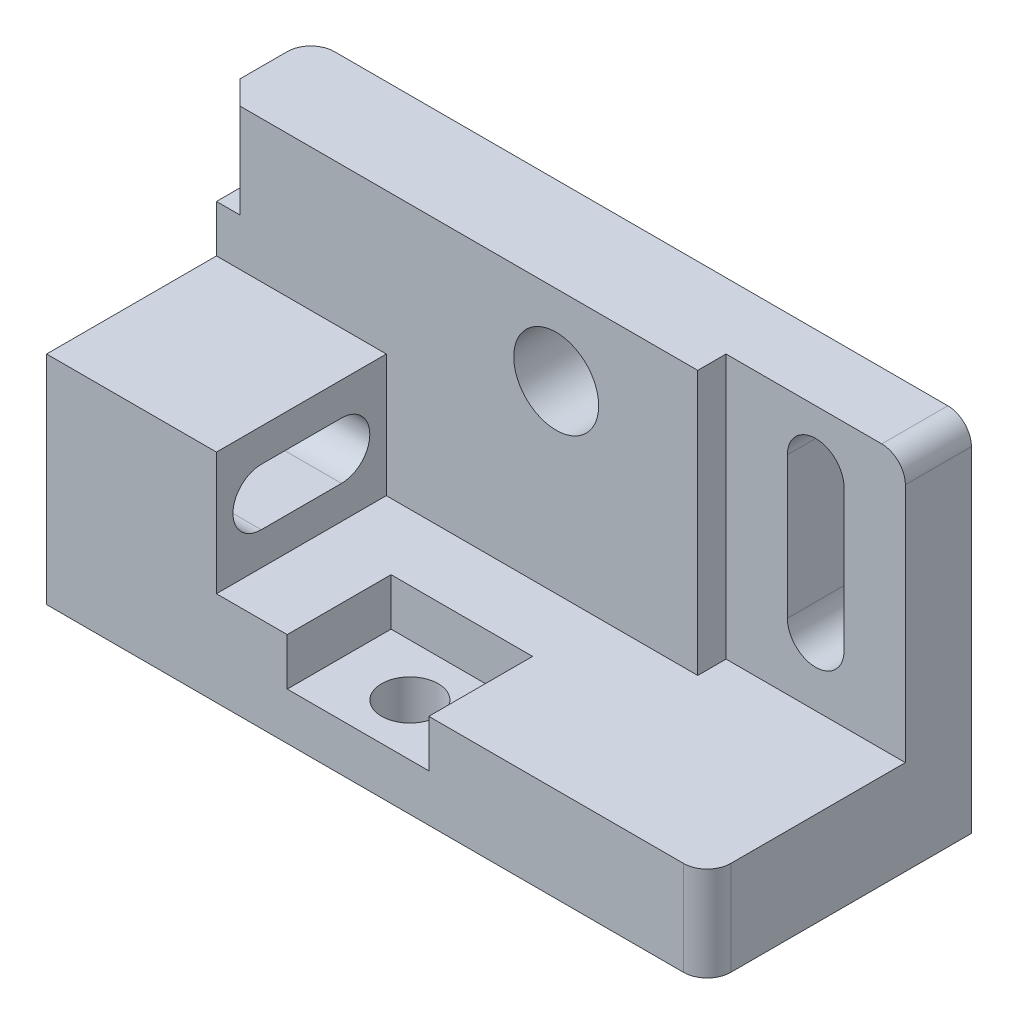
ISO-10303-21;
HEADER;
FILE_DESCRIPTION(('STEP AP214'),'2;1');
FILE_NAME('part.step','',(''),(''),'','','');
FILE_SCHEMA(('AUTOMOTIVE_DESIGN { 1 0 10303 214 1 1 1 1 }'));
ENDSEC;
DATA;
#1=APPLICATION_CONTEXT('core data for automotive mechanical design processes');
#2=APPLICATION_PROTOCOL_DEFINITION('international standard','automotive_design',2000,#1);
#3=PRODUCT_CONTEXT('',#1,'mechanical');
#4=PRODUCT('Part','Part','',(#3));
#5=PRODUCT_RELATED_PRODUCT_CATEGORY('part','',(#4));
#6=PRODUCT_DEFINITION_FORMATION('','',#4);
#7=PRODUCT_DEFINITION_CONTEXT('part definition',#1,'design');
#8=PRODUCT_DEFINITION('design','',#6,#7);
#9=PRODUCT_DEFINITION_SHAPE('','',#8);
#10=(LENGTH_UNIT() NAMED_UNIT(*) SI_UNIT(.MILLI.,.METRE.));
#11=(NAMED_UNIT(*) PLANE_ANGLE_UNIT() SI_UNIT($,.RADIAN.));
#12=(NAMED_UNIT(*) SI_UNIT($,.STERADIAN.) SOLID_ANGLE_UNIT());
#13=UNCERTAINTY_MEASURE_WITH_UNIT(LENGTH_MEASURE(1.E-05),#10,'distance_accuracy_value','');
#14=(GEOMETRIC_REPRESENTATION_CONTEXT(3) GLOBAL_UNCERTAINTY_ASSIGNED_CONTEXT((#13)) GLOBAL_UNIT_ASSIGNED_CONTEXT((#10,
#11,#12)) REPRESENTATION_CONTEXT('',''));
#15=CARTESIAN_POINT('',(0.,0.,0.));
#16=DIRECTION('',(0.,0.,1.));
#17=DIRECTION('',(1.,0.,0.));
#18=AXIS2_PLACEMENT_3D('',#15,#16,#17);
#19=CARTESIAN_POINT('',(-70.,38.,28.));
#20=DIRECTION('',(0.,-1.,0.));
#21=DIRECTION('',(0.,0.,-1.));
#22=AXIS2_PLACEMENT_3D('',#19,#20,#21);
#23=PLANE('',#22);
#24=DIRECTION('',(-1.,0.,0.));
#25=VECTOR('',#24,1.);
#26=CARTESIAN_POINT('',(70.,38.,-14.));
#27=LINE('',#26,#25);
#28=CARTESIAN_POINT('',(65.,38.,-14.));
#29=VERTEX_POINT('',#28);
#30=CARTESIAN_POINT('',(32.,38.,-14.));
#31=VERTEX_POINT('',#30);
#32=EDGE_CURVE('E337',#29,#31,#27,.T.);
#33=ORIENTED_EDGE('',*,*,#32,.F.);
#34=DIRECTION('',(0.,0.,-1.));
#35=VECTOR('',#34,1.);
#36=CARTESIAN_POINT('',(65.,38.,28.));
#37=LINE('',#36,#35);
#38=CARTESIAN_POINT('',(65.,38.,-28.));
#39=VERTEX_POINT('',#38);
#40=EDGE_CURVE('E447',#29,#39,#37,.T.);
#41=ORIENTED_EDGE('',*,*,#40,.T.);
#42=DIRECTION('',(-1.,0.,0.));
#43=VECTOR('',#42,1.);
#44=CARTESIAN_POINT('',(-70.,38.,-28.));
#45=LINE('',#44,#43);
#46=CARTESIAN_POINT('',(-65.,38.,-28.));
#47=VERTEX_POINT('',#46);
#48=EDGE_CURVE('E423',#39,#47,#45,.T.);
#49=ORIENTED_EDGE('',*,*,#48,.T.);
#50=CARTESIAN_POINT('',(-65.,38.,-23.));
#51=DIRECTION('',(0.,-1.,0.));
#52=DIRECTION('',(0.,0.,-1.));
#53=AXIS2_PLACEMENT_3D('',#50,#51,#52);
#54=CIRCLE('',#53,5.);
#55=CARTESIAN_POINT('',(-70.,38.,-23.));
#56=VERTEX_POINT('',#55);
#57=EDGE_CURVE('E271',#56,#47,#54,.T.);
#58=ORIENTED_EDGE('',*,*,#57,.F.);
#59=DIRECTION('',(0.,0.,-1.));
#60=VECTOR('',#59,1.);
#61=CARTESIAN_POINT('',(-70.,38.,28.));
#62=LINE('',#61,#60);
#63=CARTESIAN_POINT('',(-70.,38.,-13.));
#64=VERTEX_POINT('',#63);
#65=EDGE_CURVE('E431',#64,#56,#62,.T.);
#66=ORIENTED_EDGE('',*,*,#65,.F.);
#67=DIRECTION('',(-0.707106781186548,0.,-0.707106781186547));
#68=VECTOR('',#67,1.);
#69=CARTESIAN_POINT('',(-70.,38.,-13.));
#70=LINE('',#69,#68);
#71=CARTESIAN_POINT('',(-65.,38.,-8.));
#72=VERTEX_POINT('',#71);
#73=EDGE_CURVE('E279',#72,#64,#70,.T.);
#74=ORIENTED_EDGE('',*,*,#73,.F.);
#75=DIRECTION('',(-1.,0.,0.));
#76=VECTOR('',#75,1.);
#77=CARTESIAN_POINT('',(70.,38.,-8.));
#78=LINE('',#77,#76);
#79=CARTESIAN_POINT('',(32.,38.,-8.));
#80=VERTEX_POINT('',#79);
#81=EDGE_CURVE('E394',#80,#72,#78,.T.);
#82=ORIENTED_EDGE('',*,*,#81,.F.);
#83=DIRECTION('',(0.,0.,1.));
#84=VECTOR('',#83,1.);
#85=CARTESIAN_POINT('',(32.,38.,-14.));
#86=LINE('',#85,#84);
#87=EDGE_CURVE('E344',#31,#80,#86,.T.);
#88=ORIENTED_EDGE('',*,*,#87,.F.);
#89=EDGE_LOOP('',(#33,#41,#49,#58,#66,#74,#82,#88));
#90=FACE_BOUND('',#89,.T.);
#91=ADVANCED_FACE('F43',(#90),#23,.F.);
#92=CARTESIAN_POINT('',(70.,-38.,28.));
#93=DIRECTION('',(-1.,0.,0.));
#94=DIRECTION('',(0.,0.,1.));
#95=AXIS2_PLACEMENT_3D('',#92,#93,#94);
#96=PLANE('',#95);
#97=DIRECTION('',(0.,1.,0.));
#98=VECTOR('',#97,1.);
#99=CARTESIAN_POINT('',(70.,-38.,-28.));
#100=LINE('',#99,#98);
#101=CARTESIAN_POINT('',(70.,-38.,-28.));
#102=VERTEX_POINT('',#101);
#103=CARTESIAN_POINT('',(70.,33.,-28.));
#104=VERTEX_POINT('',#103);
#105=EDGE_CURVE('E409',#102,#104,#100,.T.);
#106=ORIENTED_EDGE('',*,*,#105,.T.);
#107=DIRECTION('',(0.,0.,-1.));
#108=VECTOR('',#107,1.);
#109=CARTESIAN_POINT('',(70.,33.,28.));
#110=LINE('',#109,#108);
#111=CARTESIAN_POINT('',(70.,33.,-14.));
#112=VERTEX_POINT('',#111);
#113=EDGE_CURVE('E453',#104,#112,#110,.F.);
#114=ORIENTED_EDGE('',*,*,#113,.T.);
#115=DIRECTION('',(0.,1.,0.));
#116=VECTOR('',#115,1.);
#117=CARTESIAN_POINT('',(70.,38.,-14.));
#118=LINE('',#117,#116);
#119=CARTESIAN_POINT('',(70.,-18.,-14.));
#120=VERTEX_POINT('',#119);
#121=EDGE_CURVE('E334',#120,#112,#118,.T.);
#122=ORIENTED_EDGE('',*,*,#121,.F.);
#123=DIRECTION('',(0.,0.,1.));
#124=VECTOR('',#123,1.);
#125=CARTESIAN_POINT('',(70.,-18.,-8.));
#126=LINE('',#125,#124);
#127=CARTESIAN_POINT('',(70.,-18.,23.));
#128=VERTEX_POINT('',#127);
#129=EDGE_CURVE('E404',#120,#128,#126,.T.);
#130=ORIENTED_EDGE('',*,*,#129,.T.);
#131=DIRECTION('',(0.,1.,0.));
#132=VECTOR('',#131,1.);
#133=CARTESIAN_POINT('',(70.,-38.,23.));
#134=LINE('',#133,#132);
#135=CARTESIAN_POINT('',(70.,-38.,23.));
#136=VERTEX_POINT('',#135);
#137=EDGE_CURVE('E452',#128,#136,#134,.F.);
#138=ORIENTED_EDGE('',*,*,#137,.T.);
#139=DIRECTION('',(0.,0.,-1.));
#140=VECTOR('',#139,1.);
#141=CARTESIAN_POINT('',(70.,-38.,28.));
#142=LINE('',#141,#140);
#143=EDGE_CURVE('E416',#136,#102,#142,.T.);
#144=ORIENTED_EDGE('',*,*,#143,.T.);
#145=EDGE_LOOP('',(#106,#114,#122,#130,#138,#144));
#146=FACE_BOUND('',#145,.T.);
#147=ADVANCED_FACE('F467',(#146),#96,.F.);
#148=CARTESIAN_POINT('',(-70.,-38.,28.));
#149=DIRECTION('',(1.,0.,0.));
#150=DIRECTION('',(0.,0.,-1.));
#151=AXIS2_PLACEMENT_3D('',#148,#149,#150);
#152=PLANE('',#151);
#153=DIRECTION('',(0.,0.,1.));
#154=VECTOR('',#153,1.);
#155=CARTESIAN_POINT('',(-70.,0.999999999999994,18.5));
#156=LINE('',#155,#154);
#157=CARTESIAN_POINT('',(-70.,0.999999999999994,1.5));
#158=VERTEX_POINT('',#157);
#159=CARTESIAN_POINT('',(-70.,0.999999999999994,18.5));
#160=VERTEX_POINT('',#159);
#161=EDGE_CURVE('E238',#158,#160,#156,.T.);
#162=ORIENTED_EDGE('',*,*,#161,.T.);
#163=CARTESIAN_POINT('',(-70.,-5.00000000000001,18.5));
#164=DIRECTION('',(1.,0.,0.));
#165=DIRECTION('',(0.,0.,-1.));
#166=AXIS2_PLACEMENT_3D('',#163,#164,#165);
#167=CIRCLE('',#166,6.);
#168=CARTESIAN_POINT('',(-70.,-11.,18.5));
#169=VERTEX_POINT('',#168);
#170=EDGE_CURVE('E235',#160,#169,#167,.T.);
#171=ORIENTED_EDGE('',*,*,#170,.T.);
#172=DIRECTION('',(0.,0.,-1.));
#173=VECTOR('',#172,1.);
#174=CARTESIAN_POINT('',(-70.,-11.,18.5));
#175=LINE('',#174,#173);
#176=CARTESIAN_POINT('',(-70.,-11.,1.5));
#177=VERTEX_POINT('',#176);
#178=EDGE_CURVE('E241',#169,#177,#175,.T.);
#179=ORIENTED_EDGE('',*,*,#178,.T.);
#180=CARTESIAN_POINT('',(-70.,-5.00000000000001,1.5));
#181=DIRECTION('',(1.,0.,0.));
#182=DIRECTION('',(0.,0.,-1.));
#183=AXIS2_PLACEMENT_3D('',#180,#181,#182);
#184=CIRCLE('',#183,6.);
#185=EDGE_CURVE('E248',#177,#158,#184,.T.);
#186=ORIENTED_EDGE('',*,*,#185,.T.);
#187=EDGE_LOOP('',(#162,#171,#179,#186));
#188=FACE_BOUND('',#187,.T.);
#189=DIRECTION('',(0.,0.,1.));
#190=VECTOR('',#189,1.);
#191=CARTESIAN_POINT('',(-70.,18.,-13.));
#192=LINE('',#191,#190);
#193=CARTESIAN_POINT('',(-70.,18.,-13.));
#194=VERTEX_POINT('',#193);
#195=CARTESIAN_POINT('',(-70.,18.,-8.));
#196=VERTEX_POINT('',#195);
#197=EDGE_CURVE('E274',#194,#196,#192,.T.);
#198=ORIENTED_EDGE('',*,*,#197,.F.);
#199=DIRECTION('',(0.,1.,0.));
#200=VECTOR('',#199,1.);
#201=CARTESIAN_POINT('',(-70.,18.,-13.));
#202=LINE('',#201,#200);
#203=EDGE_CURVE('E287',#194,#64,#202,.T.);
#204=ORIENTED_EDGE('',*,*,#203,.T.);
#205=ORIENTED_EDGE('',*,*,#65,.T.);
#206=DIRECTION('',(0.,1.,0.));
#207=VECTOR('',#206,1.);
#208=CARTESIAN_POINT('',(-70.,18.,-23.));
#209=LINE('',#208,#207);
#210=CARTESIAN_POINT('',(-70.,18.,-23.));
#211=VERTEX_POINT('',#210);
#212=EDGE_CURVE('E283',#211,#56,#209,.T.);
#213=ORIENTED_EDGE('',*,*,#212,.F.);
#214=DIRECTION('',(0.,0.,1.));
#215=VECTOR('',#214,1.);
#216=CARTESIAN_POINT('',(-70.,18.,-23.));
#217=LINE('',#216,#215);
#218=CARTESIAN_POINT('',(-70.,18.,-28.));
#219=VERTEX_POINT('',#218);
#220=EDGE_CURVE('E293',#219,#211,#217,.T.);
#221=ORIENTED_EDGE('',*,*,#220,.F.);
#222=DIRECTION('',(0.,-1.,0.));
#223=VECTOR('',#222,1.);
#224=CARTESIAN_POINT('',(-70.,-38.,-28.));
#225=LINE('',#224,#223);
#226=CARTESIAN_POINT('',(-70.,-38.,-28.));
#227=VERTEX_POINT('',#226);
#228=EDGE_CURVE('E421',#219,#227,#225,.T.);
#229=ORIENTED_EDGE('',*,*,#228,.T.);
#230=DIRECTION('',(0.,0.,-1.));
#231=VECTOR('',#230,1.);
#232=CARTESIAN_POINT('',(-70.,-38.,28.));
#233=LINE('',#232,#231);
#234=CARTESIAN_POINT('',(-70.,-38.,28.));
#235=VERTEX_POINT('',#234);
#236=EDGE_CURVE('E428',#235,#227,#233,.T.);
#237=ORIENTED_EDGE('',*,*,#236,.F.);
#238=DIRECTION('',(0.,-1.,0.));
#239=VECTOR('',#238,1.);
#240=CARTESIAN_POINT('',(-70.,-38.,28.));
#241=LINE('',#240,#239);
#242=CARTESIAN_POINT('',(-70.,7.99999999999999,28.));
#243=VERTEX_POINT('',#242);
#244=EDGE_CURVE('E413',#243,#235,#241,.T.);
#245=ORIENTED_EDGE('',*,*,#244,.F.);
#246=DIRECTION('',(0.,0.,1.));
#247=VECTOR('',#246,1.);
#248=CARTESIAN_POINT('',(-70.,7.99999999999999,-8.));
#249=LINE('',#248,#247);
#250=CARTESIAN_POINT('',(-70.,7.99999999999999,-8.));
#251=VERTEX_POINT('',#250);
#252=EDGE_CURVE('E393',#251,#243,#249,.T.);
#253=ORIENTED_EDGE('',*,*,#252,.F.);
#254=DIRECTION('',(0.,-1.,0.));
#255=VECTOR('',#254,1.);
#256=CARTESIAN_POINT('',(-70.,38.,-8.));
#257=LINE('',#256,#255);
#258=EDGE_CURVE('E379',#196,#251,#257,.T.);
#259=ORIENTED_EDGE('',*,*,#258,.F.);
#260=EDGE_LOOP('',(#198,#204,#205,#213,#221,#229,#237,#245,#253,#259));
#261=FACE_BOUND('',#260,.T.);
#262=ADVANCED_FACE('F246',(#188,#261),#152,.F.);
#263=CARTESIAN_POINT('',(-70.,-38.,28.));
#264=DIRECTION('',(0.,1.,0.));
#265=DIRECTION('',(0.,0.,1.));
#266=AXIS2_PLACEMENT_3D('',#263,#264,#265);
#267=PLANE('',#266);
#268=CARTESIAN_POINT('',(-4.00000000000002,-38.,17.));
#269=DIRECTION('',(0.,1.,0.));
#270=DIRECTION('',(0.,0.,1.));
#271=AXIS2_PLACEMENT_3D('',#268,#269,#270);
#272=CIRCLE('',#271,6.);
#273=CARTESIAN_POINT('',(-4.00000000000002,-38.,23.));
#274=VERTEX_POINT('',#273);
#275=EDGE_CURVE('E259',#274,#274,#272,.T.);
#276=ORIENTED_EDGE('',*,*,#275,.T.);
#277=EDGE_LOOP('',(#276));
#278=FACE_BOUND('',#277,.T.);
#279=ORIENTED_EDGE('',*,*,#143,.F.);
#280=CARTESIAN_POINT('',(65.,-38.,23.));
#281=DIRECTION('',(0.,1.,0.));
#282=DIRECTION('',(0.,0.,1.));
#283=AXIS2_PLACEMENT_3D('',#280,#281,#282);
#284=CIRCLE('',#283,5.);
#285=CARTESIAN_POINT('',(65.,-38.,28.));
#286=VERTEX_POINT('',#285);
#287=EDGE_CURVE('E11',#136,#286,#284,.F.);
#288=ORIENTED_EDGE('',*,*,#287,.T.);
#289=DIRECTION('',(1.,0.,0.));
#290=VECTOR('',#289,1.);
#291=CARTESIAN_POINT('',(-70.,-38.,28.));
#292=LINE('',#291,#290);
#293=EDGE_CURVE('E411',#235,#286,#292,.T.);
#294=ORIENTED_EDGE('',*,*,#293,.F.);
#295=ORIENTED_EDGE('',*,*,#236,.T.);
#296=DIRECTION('',(1.,0.,0.));
#297=VECTOR('',#296,1.);
#298=CARTESIAN_POINT('',(-70.,-38.,-28.));
#299=LINE('',#298,#297);
#300=EDGE_CURVE('E418',#227,#102,#299,.T.);
#301=ORIENTED_EDGE('',*,*,#300,.T.);
#302=EDGE_LOOP('',(#279,#288,#294,#295,#301));
#303=FACE_BOUND('',#302,.T.);
#304=ADVANCED_FACE('F471',(#278,#303),#267,.F.);
#305=CARTESIAN_POINT('',(0.,0.,28.));
#306=DIRECTION('',(0.,0.,-1.));
#307=DIRECTION('',(-1.,0.,0.));
#308=AXIS2_PLACEMENT_3D('',#305,#306,#307);
#309=PLANE('',#308);
#310=ORIENTED_EDGE('',*,*,#293,.T.);
#311=DIRECTION('',(0.,1.,0.));
#312=VECTOR('',#311,1.);
#313=CARTESIAN_POINT('',(65.,0.,28.));
#314=LINE('',#313,#312);
#315=CARTESIAN_POINT('',(65.,-18.,28.));
#316=VERTEX_POINT('',#315);
#317=EDGE_CURVE('E460',#286,#316,#314,.T.);
#318=ORIENTED_EDGE('',*,*,#317,.T.);
#319=DIRECTION('',(1.,0.,0.));
#320=VECTOR('',#319,1.);
#321=CARTESIAN_POINT('',(-34.,-18.,28.));
#322=LINE('',#321,#320);
#323=CARTESIAN_POINT('',(11.,-18.,28.));
#324=VERTEX_POINT('',#323);
#325=EDGE_CURVE('E402',#324,#316,#322,.T.);
#326=ORIENTED_EDGE('',*,*,#325,.F.);
#327=DIRECTION('',(0.,1.,0.));
#328=VECTOR('',#327,1.);
#329=CARTESIAN_POINT('',(11.,-28.,28.));
#330=LINE('',#329,#328);
#331=CARTESIAN_POINT('',(11.,-28.,28.));
#332=VERTEX_POINT('',#331);
#333=EDGE_CURVE('E367',#332,#324,#330,.T.);
#334=ORIENTED_EDGE('',*,*,#333,.F.);
#335=DIRECTION('',(1.,0.,0.));
#336=VECTOR('',#335,1.);
#337=CARTESIAN_POINT('',(11.,-28.,28.));
#338=LINE('',#337,#336);
#339=CARTESIAN_POINT('',(-19.,-28.,28.));
#340=VERTEX_POINT('',#339);
#341=EDGE_CURVE('E363',#340,#332,#338,.T.);
#342=ORIENTED_EDGE('',*,*,#341,.F.);
#343=DIRECTION('',(0.,1.,0.));
#344=VECTOR('',#343,1.);
#345=CARTESIAN_POINT('',(-19.,-28.,28.));
#346=LINE('',#345,#344);
#347=CARTESIAN_POINT('',(-19.,-18.,28.));
#348=VERTEX_POINT('',#347);
#349=EDGE_CURVE('E373',#340,#348,#346,.T.);
#350=ORIENTED_EDGE('',*,*,#349,.T.);
#351=CARTESIAN_POINT('',(-34.,-18.,28.));
#352=VERTEX_POINT('',#351);
#353=EDGE_CURVE('E382',#352,#348,#322,.T.);
#354=ORIENTED_EDGE('',*,*,#353,.F.);
#355=DIRECTION('',(0.,-1.,0.));
#356=VECTOR('',#355,1.);
#357=CARTESIAN_POINT('',(-34.,7.99999999999999,28.));
#358=LINE('',#357,#356);
#359=CARTESIAN_POINT('',(-34.,7.99999999999999,28.));
#360=VERTEX_POINT('',#359);
#361=EDGE_CURVE('E398',#360,#352,#358,.T.);
#362=ORIENTED_EDGE('',*,*,#361,.F.);
#363=DIRECTION('',(1.,0.,0.));
#364=VECTOR('',#363,1.);
#365=CARTESIAN_POINT('',(-70.,7.99999999999999,28.));
#366=LINE('',#365,#364);
#367=EDGE_CURVE('E375',#243,#360,#366,.T.);
#368=ORIENTED_EDGE('',*,*,#367,.F.);
#369=ORIENTED_EDGE('',*,*,#244,.T.);
#370=EDGE_LOOP('',(#310,#318,#326,#334,#342,#350,#354,#362,#368,#369));
#371=FACE_BOUND('',#370,.T.);
#372=ADVANCED_FACE('F468',(#371),#309,.F.);
#373=CARTESIAN_POINT('',(0.,0.,-28.));
#374=DIRECTION('',(0.,0.,-1.));
#375=DIRECTION('',(-1.,0.,0.));
#376=AXIS2_PLACEMENT_3D('',#373,#374,#375);
#377=PLANE('',#376);
#378=ORIENTED_EDGE('',*,*,#48,.F.);
#379=CARTESIAN_POINT('',(65.,33.,-28.));
#380=DIRECTION('',(0.,0.,-1.));
#381=DIRECTION('',(-1.,0.,0.));
#382=AXIS2_PLACEMENT_3D('',#379,#380,#381);
#383=CIRCLE('',#382,5.);
#384=EDGE_CURVE('E446',#39,#104,#383,.T.);
#385=ORIENTED_EDGE('',*,*,#384,.T.);
#386=ORIENTED_EDGE('',*,*,#105,.F.);
#387=ORIENTED_EDGE('',*,*,#300,.F.);
#388=ORIENTED_EDGE('',*,*,#228,.F.);
#389=DIRECTION('',(-1.,0.,0.));
#390=VECTOR('',#389,1.);
#391=CARTESIAN_POINT('',(-70.,18.,-28.));
#392=LINE('',#391,#390);
#393=CARTESIAN_POINT('',(-65.,18.,-28.));
#394=VERTEX_POINT('',#393);
#395=EDGE_CURVE('E291',#394,#219,#392,.T.);
#396=ORIENTED_EDGE('',*,*,#395,.F.);
#397=DIRECTION('',(0.,1.,0.));
#398=VECTOR('',#397,1.);
#399=CARTESIAN_POINT('',(-65.,18.,-28.));
#400=LINE('',#399,#398);
#401=EDGE_CURVE('E300',#394,#47,#400,.T.);
#402=ORIENTED_EDGE('',*,*,#401,.T.);
#403=EDGE_LOOP('',(#378,#385,#386,#387,#388,#396,#402));
#404=FACE_BOUND('',#403,.T.);
#405=CARTESIAN_POINT('',(1.99999999999999,21.,-28.));
#406=DIRECTION('',(0.,0.,1.));
#407=DIRECTION('',(1.,0.,0.));
#408=AXIS2_PLACEMENT_3D('',#405,#406,#407);
#409=CIRCLE('',#408,9.);
#410=CARTESIAN_POINT('',(11.,21.,-28.));
#411=VERTEX_POINT('',#410);
#412=EDGE_CURVE('E304',#411,#411,#409,.T.);
#413=ORIENTED_EDGE('',*,*,#412,.T.);
#414=EDGE_LOOP('',(#413));
#415=FACE_BOUND('',#414,.T.);
#416=CARTESIAN_POINT('',(51.,-4.00000000000001,-28.));
#417=DIRECTION('',(0.,0.,1.));
#418=DIRECTION('',(1.,0.,0.));
#419=AXIS2_PLACEMENT_3D('',#416,#417,#418);
#420=CIRCLE('',#419,6.);
#421=CARTESIAN_POINT('',(45.,-4.00000000000001,-28.));
#422=VERTEX_POINT('',#421);
#423=CARTESIAN_POINT('',(57.,-4.00000000000001,-28.));
#424=VERTEX_POINT('',#423);
#425=EDGE_CURVE('E289',#422,#424,#420,.T.);
#426=ORIENTED_EDGE('',*,*,#425,.T.);
#427=DIRECTION('',(0.,1.,0.));
#428=VECTOR('',#427,1.);
#429=CARTESIAN_POINT('',(57.,-4.00000000000001,-28.));
#430=LINE('',#429,#428);
#431=CARTESIAN_POINT('',(57.,26.,-28.));
#432=VERTEX_POINT('',#431);
#433=EDGE_CURVE('E314',#424,#432,#430,.T.);
#434=ORIENTED_EDGE('',*,*,#433,.T.);
#435=CARTESIAN_POINT('',(51.,26.,-28.));
#436=DIRECTION('',(0.,0.,1.));
#437=DIRECTION('',(1.,0.,0.));
#438=AXIS2_PLACEMENT_3D('',#435,#436,#437);
#439=CIRCLE('',#438,6.);
#440=CARTESIAN_POINT('',(45.,26.,-28.));
#441=VERTEX_POINT('',#440);
#442=EDGE_CURVE('E320',#432,#441,#439,.T.);
#443=ORIENTED_EDGE('',*,*,#442,.T.);
#444=DIRECTION('',(0.,-1.,0.));
#445=VECTOR('',#444,1.);
#446=CARTESIAN_POINT('',(45.,-4.00000000000001,-28.));
#447=LINE('',#446,#445);
#448=EDGE_CURVE('E319',#441,#422,#447,.T.);
#449=ORIENTED_EDGE('',*,*,#448,.T.);
#450=EDGE_LOOP('',(#426,#434,#443,#449));
#451=FACE_BOUND('',#450,.T.);
#452=ADVANCED_FACE('F479',(#404,#415,#451),#377,.T.);
#453=CARTESIAN_POINT('',(-34.,-18.,-8.));
#454=DIRECTION('',(0.,-1.,0.));
#455=DIRECTION('',(0.,0.,-1.));
#456=AXIS2_PLACEMENT_3D('',#453,#454,#455);
#457=PLANE('',#456);
#458=ORIENTED_EDGE('',*,*,#325,.T.);
#459=CARTESIAN_POINT('',(65.,-18.,23.));
#460=DIRECTION('',(0.,-1.,0.));
#461=DIRECTION('',(0.,0.,-1.));
#462=AXIS2_PLACEMENT_3D('',#459,#460,#461);
#463=CIRCLE('',#462,5.);
#464=EDGE_CURVE('E51',#316,#128,#463,.F.);
#465=ORIENTED_EDGE('',*,*,#464,.T.);
#466=ORIENTED_EDGE('',*,*,#129,.F.);
#467=DIRECTION('',(1.,0.,0.));
#468=VECTOR('',#467,1.);
#469=CARTESIAN_POINT('',(70.,-18.,-14.));
#470=LINE('',#469,#468);
#471=CARTESIAN_POINT('',(32.,-18.,-14.));
#472=VERTEX_POINT('',#471);
#473=EDGE_CURVE('E342',#472,#120,#470,.T.);
#474=ORIENTED_EDGE('',*,*,#473,.F.);
#475=DIRECTION('',(0.,0.,1.));
#476=VECTOR('',#475,1.);
#477=CARTESIAN_POINT('',(32.,-18.,-14.));
#478=LINE('',#477,#476);
#479=CARTESIAN_POINT('',(32.,-18.,-8.));
#480=VERTEX_POINT('',#479);
#481=EDGE_CURVE('E350',#472,#480,#478,.T.);
#482=ORIENTED_EDGE('',*,*,#481,.T.);
#483=DIRECTION('',(1.,0.,0.));
#484=VECTOR('',#483,1.);
#485=CARTESIAN_POINT('',(-34.,-18.,-8.));
#486=LINE('',#485,#484);
#487=CARTESIAN_POINT('',(-34.,-18.,-8.));
#488=VERTEX_POINT('',#487);
#489=EDGE_CURVE('E386',#488,#480,#486,.T.);
#490=ORIENTED_EDGE('',*,*,#489,.F.);
#491=DIRECTION('',(0.,0.,1.));
#492=VECTOR('',#491,1.);
#493=CARTESIAN_POINT('',(-34.,-18.,-8.));
#494=LINE('',#493,#492);
#495=EDGE_CURVE('E410',#488,#352,#494,.T.);
#496=ORIENTED_EDGE('',*,*,#495,.T.);
#497=ORIENTED_EDGE('',*,*,#353,.T.);
#498=DIRECTION('',(0.,0.,1.));
#499=VECTOR('',#498,1.);
#500=CARTESIAN_POINT('',(-19.,-18.,28.));
#501=LINE('',#500,#499);
#502=CARTESIAN_POINT('',(-19.,-18.,6.00000000000001));
#503=VERTEX_POINT('',#502);
#504=EDGE_CURVE('E353',#503,#348,#501,.T.);
#505=ORIENTED_EDGE('',*,*,#504,.F.);
#506=DIRECTION('',(-1.,0.,0.));
#507=VECTOR('',#506,1.);
#508=CARTESIAN_POINT('',(11.,-18.,6.));
#509=LINE('',#508,#507);
#510=CARTESIAN_POINT('',(11.,-18.,6.));
#511=VERTEX_POINT('',#510);
#512=EDGE_CURVE('E368',#511,#503,#509,.T.);
#513=ORIENTED_EDGE('',*,*,#512,.F.);
#514=DIRECTION('',(0.,0.,-1.));
#515=VECTOR('',#514,1.);
#516=CARTESIAN_POINT('',(11.,-18.,28.));
#517=LINE('',#516,#515);
#518=EDGE_CURVE('E349',#324,#511,#517,.T.);
#519=ORIENTED_EDGE('',*,*,#518,.F.);
#520=EDGE_LOOP('',(#458,#465,#466,#474,#482,#490,#496,#497,#505,#513,#519));
#521=FACE_BOUND('',#520,.T.);
#522=ADVANCED_FACE('F458',(#521),#457,.F.);
#523=CARTESIAN_POINT('',(-34.,7.99999999999999,-8.));
#524=DIRECTION('',(-1.,0.,0.));
#525=DIRECTION('',(0.,0.,1.));
#526=AXIS2_PLACEMENT_3D('',#523,#524,#525);
#527=PLANE('',#526);
#528=DIRECTION('',(0.,0.,-1.));
#529=VECTOR('',#528,1.);
#530=CARTESIAN_POINT('',(-34.,-11.,18.5));
#531=LINE('',#530,#529);
#532=CARTESIAN_POINT('',(-34.,-11.,18.5));
#533=VERTEX_POINT('',#532);
#534=CARTESIAN_POINT('',(-34.,-11.,1.5));
#535=VERTEX_POINT('',#534);
#536=EDGE_CURVE('E264',#533,#535,#531,.T.);
#537=ORIENTED_EDGE('',*,*,#536,.F.);
#538=CARTESIAN_POINT('',(-34.,-5.00000000000001,18.5));
#539=DIRECTION('',(1.,0.,0.));
#540=DIRECTION('',(0.,0.,-1.));
#541=AXIS2_PLACEMENT_3D('',#538,#539,#540);
#542=CIRCLE('',#541,6.);
#543=CARTESIAN_POINT('',(-34.,0.999999999999994,18.5));
#544=VERTEX_POINT('',#543);
#545=EDGE_CURVE('E231',#544,#533,#542,.T.);
#546=ORIENTED_EDGE('',*,*,#545,.F.);
#547=DIRECTION('',(0.,0.,1.));
#548=VECTOR('',#547,1.);
#549=CARTESIAN_POINT('',(-34.,0.999999999999994,18.5));
#550=LINE('',#549,#548);
#551=CARTESIAN_POINT('',(-34.,0.999999999999994,1.5));
#552=VERTEX_POINT('',#551);
#553=EDGE_CURVE('E251',#552,#544,#550,.T.);
#554=ORIENTED_EDGE('',*,*,#553,.F.);
#555=CARTESIAN_POINT('',(-34.,-5.00000000000001,1.5));
#556=DIRECTION('',(1.,0.,0.));
#557=DIRECTION('',(0.,0.,-1.));
#558=AXIS2_PLACEMENT_3D('',#555,#556,#557);
#559=CIRCLE('',#558,6.);
#560=EDGE_CURVE('E258',#535,#552,#559,.T.);
#561=ORIENTED_EDGE('',*,*,#560,.F.);
#562=EDGE_LOOP('',(#537,#546,#554,#561));
#563=FACE_BOUND('',#562,.T.);
#564=ORIENTED_EDGE('',*,*,#361,.T.);
#565=ORIENTED_EDGE('',*,*,#495,.F.);
#566=DIRECTION('',(0.,-1.,0.));
#567=VECTOR('',#566,1.);
#568=CARTESIAN_POINT('',(-34.,7.99999999999999,-8.));
#569=LINE('',#568,#567);
#570=CARTESIAN_POINT('',(-34.,7.99999999999999,-8.));
#571=VERTEX_POINT('',#570);
#572=EDGE_CURVE('E387',#571,#488,#569,.T.);
#573=ORIENTED_EDGE('',*,*,#572,.F.);
#574=DIRECTION('',(0.,0.,1.));
#575=VECTOR('',#574,1.);
#576=CARTESIAN_POINT('',(-34.,7.99999999999999,-8.));
#577=LINE('',#576,#575);
#578=EDGE_CURVE('E408',#571,#360,#577,.T.);
#579=ORIENTED_EDGE('',*,*,#578,.T.);
#580=EDGE_LOOP('',(#564,#565,#573,#579));
#581=FACE_BOUND('',#580,.T.);
#582=ADVANCED_FACE('F508',(#563,#581),#527,.F.);
#583=CARTESIAN_POINT('',(-70.,7.99999999999999,-8.));
#584=DIRECTION('',(0.,-1.,0.));
#585=DIRECTION('',(0.,0.,-1.));
#586=AXIS2_PLACEMENT_3D('',#583,#584,#585);
#587=PLANE('',#586);
#588=ORIENTED_EDGE('',*,*,#367,.T.);
#589=ORIENTED_EDGE('',*,*,#578,.F.);
#590=DIRECTION('',(1.,0.,0.));
#591=VECTOR('',#590,1.);
#592=CARTESIAN_POINT('',(-70.,7.99999999999999,-8.));
#593=LINE('',#592,#591);
#594=EDGE_CURVE('E385',#251,#571,#593,.T.);
#595=ORIENTED_EDGE('',*,*,#594,.F.);
#596=ORIENTED_EDGE('',*,*,#252,.T.);
#597=EDGE_LOOP('',(#588,#589,#595,#596));
#598=FACE_BOUND('',#597,.T.);
#599=ADVANCED_FACE('F530',(#598),#587,.F.);
#600=CARTESIAN_POINT('',(0.,0.,-8.));
#601=DIRECTION('',(0.,0.,1.));
#602=DIRECTION('',(1.,0.,0.));
#603=AXIS2_PLACEMENT_3D('',#600,#601,#602);
#604=PLANE('',#603);
#605=DIRECTION('',(0.,1.,0.));
#606=VECTOR('',#605,1.);
#607=CARTESIAN_POINT('',(-65.,18.,-8.));
#608=LINE('',#607,#606);
#609=CARTESIAN_POINT('',(-65.,18.,-8.));
#610=VERTEX_POINT('',#609);
#611=EDGE_CURVE('E285',#610,#72,#608,.T.);
#612=ORIENTED_EDGE('',*,*,#611,.F.);
#613=DIRECTION('',(1.,0.,0.));
#614=VECTOR('',#613,1.);
#615=CARTESIAN_POINT('',(-70.,18.,-8.));
#616=LINE('',#615,#614);
#617=EDGE_CURVE('E280',#196,#610,#616,.T.);
#618=ORIENTED_EDGE('',*,*,#617,.F.);
#619=ORIENTED_EDGE('',*,*,#258,.T.);
#620=ORIENTED_EDGE('',*,*,#594,.T.);
#621=ORIENTED_EDGE('',*,*,#572,.T.);
#622=ORIENTED_EDGE('',*,*,#489,.T.);
#623=DIRECTION('',(0.,-1.,0.));
#624=VECTOR('',#623,1.);
#625=CARTESIAN_POINT('',(32.,38.,-8.));
#626=LINE('',#625,#624);
#627=EDGE_CURVE('E307',#80,#480,#626,.T.);
#628=ORIENTED_EDGE('',*,*,#627,.F.);
#629=ORIENTED_EDGE('',*,*,#81,.T.);
#630=EDGE_LOOP('',(#612,#618,#619,#620,#621,#622,#628,#629));
#631=FACE_BOUND('',#630,.T.);
#632=CARTESIAN_POINT('',(1.99999999999999,21.,-8.));
#633=DIRECTION('',(0.,0.,1.));
#634=DIRECTION('',(1.,0.,0.));
#635=AXIS2_PLACEMENT_3D('',#632,#633,#634);
#636=CIRCLE('',#635,9.);
#637=CARTESIAN_POINT('',(11.,21.,-8.));
#638=VERTEX_POINT('',#637);
#639=EDGE_CURVE('E306',#638,#638,#636,.T.);
#640=ORIENTED_EDGE('',*,*,#639,.F.);
#641=EDGE_LOOP('',(#640));
#642=FACE_BOUND('',#641,.T.);
#643=ADVANCED_FACE('F498',(#631,#642),#604,.T.);
#644=CARTESIAN_POINT('',(11.,-28.,28.));
#645=DIRECTION('',(1.,0.,0.));
#646=DIRECTION('',(0.,0.,-1.));
#647=AXIS2_PLACEMENT_3D('',#644,#645,#646);
#648=PLANE('',#647);
#649=ORIENTED_EDGE('',*,*,#518,.T.);
#650=DIRECTION('',(0.,1.,0.));
#651=VECTOR('',#650,1.);
#652=CARTESIAN_POINT('',(11.,-28.,6.));
#653=LINE('',#652,#651);
#654=CARTESIAN_POINT('',(11.,-28.,6.));
#655=VERTEX_POINT('',#654);
#656=EDGE_CURVE('E365',#655,#511,#653,.T.);
#657=ORIENTED_EDGE('',*,*,#656,.F.);
#658=DIRECTION('',(0.,0.,-1.));
#659=VECTOR('',#658,1.);
#660=CARTESIAN_POINT('',(11.,-28.,28.));
#661=LINE('',#660,#659);
#662=EDGE_CURVE('E352',#332,#655,#661,.T.);
#663=ORIENTED_EDGE('',*,*,#662,.F.);
#664=ORIENTED_EDGE('',*,*,#333,.T.);
#665=EDGE_LOOP('',(#649,#657,#663,#664));
#666=FACE_BOUND('',#665,.T.);
#667=ADVANCED_FACE('F518',(#666),#648,.F.);
#668=CARTESIAN_POINT('',(-19.,-28.,28.));
#669=DIRECTION('',(-1.,0.,0.));
#670=DIRECTION('',(0.,0.,1.));
#671=AXIS2_PLACEMENT_3D('',#668,#669,#670);
#672=PLANE('',#671);
#673=ORIENTED_EDGE('',*,*,#504,.T.);
#674=ORIENTED_EDGE('',*,*,#349,.F.);
#675=DIRECTION('',(0.,0.,1.));
#676=VECTOR('',#675,1.);
#677=CARTESIAN_POINT('',(-19.,-28.,28.));
#678=LINE('',#677,#676);
#679=CARTESIAN_POINT('',(-19.,-28.,6.00000000000001));
#680=VERTEX_POINT('',#679);
#681=EDGE_CURVE('E358',#680,#340,#678,.T.);
#682=ORIENTED_EDGE('',*,*,#681,.F.);
#683=DIRECTION('',(0.,1.,0.));
#684=VECTOR('',#683,1.);
#685=CARTESIAN_POINT('',(-19.,-28.,6.00000000000001));
#686=LINE('',#685,#684);
#687=EDGE_CURVE('E376',#680,#503,#686,.T.);
#688=ORIENTED_EDGE('',*,*,#687,.T.);
#689=EDGE_LOOP('',(#673,#674,#682,#688));
#690=FACE_BOUND('',#689,.T.);
#691=ADVANCED_FACE('F515',(#690),#672,.F.);
#692=CARTESIAN_POINT('',(11.,-28.,6.));
#693=DIRECTION('',(0.,0.,-1.));
#694=DIRECTION('',(-1.,0.,0.));
#695=AXIS2_PLACEMENT_3D('',#692,#693,#694);
#696=PLANE('',#695);
#697=ORIENTED_EDGE('',*,*,#512,.T.);
#698=ORIENTED_EDGE('',*,*,#687,.F.);
#699=DIRECTION('',(-1.,0.,0.));
#700=VECTOR('',#699,1.);
#701=CARTESIAN_POINT('',(11.,-28.,6.));
#702=LINE('',#701,#700);
#703=EDGE_CURVE('E351',#655,#680,#702,.T.);
#704=ORIENTED_EDGE('',*,*,#703,.F.);
#705=ORIENTED_EDGE('',*,*,#656,.T.);
#706=EDGE_LOOP('',(#697,#698,#704,#705));
#707=FACE_BOUND('',#706,.T.);
#708=ADVANCED_FACE('F519',(#707),#696,.F.);
#709=CARTESIAN_POINT('',(0.,-28.,0.));
#710=DIRECTION('',(0.,1.,0.));
#711=DIRECTION('',(0.,0.,1.));
#712=AXIS2_PLACEMENT_3D('',#709,#710,#711);
#713=PLANE('',#712);
#714=CARTESIAN_POINT('',(-4.00000000000002,-28.,17.));
#715=DIRECTION('',(0.,1.,0.));
#716=DIRECTION('',(0.,0.,1.));
#717=AXIS2_PLACEMENT_3D('',#714,#715,#716);
#718=CIRCLE('',#717,6.);
#719=CARTESIAN_POINT('',(-4.00000000000002,-28.,23.));
#720=VERTEX_POINT('',#719);
#721=EDGE_CURVE('E854',#720,#720,#718,.T.);
#722=ORIENTED_EDGE('',*,*,#721,.F.);
#723=EDGE_LOOP('',(#722));
#724=FACE_BOUND('',#723,.T.);
#725=ORIENTED_EDGE('',*,*,#662,.T.);
#726=ORIENTED_EDGE('',*,*,#703,.T.);
#727=ORIENTED_EDGE('',*,*,#681,.T.);
#728=ORIENTED_EDGE('',*,*,#341,.T.);
#729=EDGE_LOOP('',(#725,#726,#727,#728));
#730=FACE_BOUND('',#729,.T.);
#731=ADVANCED_FACE('F514',(#724,#730),#713,.T.);
#732=CARTESIAN_POINT('',(32.,38.,-14.));
#733=DIRECTION('',(-1.,0.,0.));
#734=DIRECTION('',(0.,-1.,0.));
#735=AXIS2_PLACEMENT_3D('',#732,#733,#734);
#736=PLANE('',#735);
#737=ORIENTED_EDGE('',*,*,#627,.T.);
#738=ORIENTED_EDGE('',*,*,#481,.F.);
#739=DIRECTION('',(0.,-1.,0.));
#740=VECTOR('',#739,1.);
#741=CARTESIAN_POINT('',(32.,38.,-14.));
#742=LINE('',#741,#740);
#743=EDGE_CURVE('E340',#31,#472,#742,.T.);
#744=ORIENTED_EDGE('',*,*,#743,.F.);
#745=ORIENTED_EDGE('',*,*,#87,.T.);
#746=EDGE_LOOP('',(#737,#738,#744,#745));
#747=FACE_BOUND('',#746,.T.);
#748=ADVANCED_FACE('F500',(#747),#736,.F.);
#749=CARTESIAN_POINT('',(0.,0.,-14.));
#750=DIRECTION('',(0.,0.,-1.));
#751=DIRECTION('',(-1.,0.,0.));
#752=AXIS2_PLACEMENT_3D('',#749,#750,#751);
#753=PLANE('',#752);
#754=DIRECTION('',(0.,-1.,0.));
#755=VECTOR('',#754,1.);
#756=CARTESIAN_POINT('',(57.,0.,-14.));
#757=LINE('',#756,#755);
#758=CARTESIAN_POINT('',(57.,26.,-14.));
#759=VERTEX_POINT('',#758);
#760=CARTESIAN_POINT('',(57.,-4.00000000000001,-14.));
#761=VERTEX_POINT('',#760);
#762=EDGE_CURVE('E432',#759,#761,#757,.T.);
#763=ORIENTED_EDGE('',*,*,#762,.T.);
#764=CARTESIAN_POINT('',(51.,-4.00000000000001,-14.));
#765=DIRECTION('',(0.,0.,-1.));
#766=DIRECTION('',(-1.,0.,0.));
#767=AXIS2_PLACEMENT_3D('',#764,#765,#766);
#768=CIRCLE('',#767,6.);
#769=CARTESIAN_POINT('',(45.,-4.00000000000001,-14.));
#770=VERTEX_POINT('',#769);
#771=EDGE_CURVE('E444',#761,#770,#768,.T.);
#772=ORIENTED_EDGE('',*,*,#771,.T.);
#773=DIRECTION('',(0.,1.,0.));
#774=VECTOR('',#773,1.);
#775=CARTESIAN_POINT('',(45.,0.,-14.));
#776=LINE('',#775,#774);
#777=CARTESIAN_POINT('',(45.,26.,-14.));
#778=VERTEX_POINT('',#777);
#779=EDGE_CURVE('E439',#770,#778,#776,.T.);
#780=ORIENTED_EDGE('',*,*,#779,.T.);
#781=CARTESIAN_POINT('',(51.,26.,-14.));
#782=DIRECTION('',(0.,0.,-1.));
#783=DIRECTION('',(-1.,0.,0.));
#784=AXIS2_PLACEMENT_3D('',#781,#782,#783);
#785=CIRCLE('',#784,6.);
#786=EDGE_CURVE('E440',#778,#759,#785,.T.);
#787=ORIENTED_EDGE('',*,*,#786,.T.);
#788=EDGE_LOOP('',(#763,#772,#780,#787));
#789=FACE_BOUND('',#788,.T.);
#790=ORIENTED_EDGE('',*,*,#121,.T.);
#791=CARTESIAN_POINT('',(65.,33.,-14.));
#792=DIRECTION('',(0.,0.,-1.));
#793=DIRECTION('',(-1.,0.,0.));
#794=AXIS2_PLACEMENT_3D('',#791,#792,#793);
#795=CIRCLE('',#794,5.);
#796=EDGE_CURVE('E451',#112,#29,#795,.F.);
#797=ORIENTED_EDGE('',*,*,#796,.T.);
#798=ORIENTED_EDGE('',*,*,#32,.T.);
#799=ORIENTED_EDGE('',*,*,#743,.T.);
#800=ORIENTED_EDGE('',*,*,#473,.T.);
#801=EDGE_LOOP('',(#790,#797,#798,#799,#800));
#802=FACE_BOUND('',#801,.T.);
#803=ADVANCED_FACE('F487',(#789,#802),#753,.F.);
#804=CARTESIAN_POINT('',(51.,-4.00000000000001,-28.));
#805=DIRECTION('',(0.,0.,1.));
#806=DIRECTION('',(1.,0.,0.));
#807=AXIS2_PLACEMENT_3D('',#804,#805,#806);
#808=CYLINDRICAL_SURFACE('',#807,6.);
#809=DIRECTION('',(0.,0.,1.));
#810=VECTOR('',#809,1.);
#811=CARTESIAN_POINT('',(57.,-4.00000000000001,-28.));
#812=LINE('',#811,#810);
#813=EDGE_CURVE('E323',#424,#761,#812,.T.);
#814=ORIENTED_EDGE('',*,*,#813,.F.);
#815=ORIENTED_EDGE('',*,*,#425,.F.);
#816=DIRECTION('',(0.,0.,1.));
#817=VECTOR('',#816,1.);
#818=CARTESIAN_POINT('',(45.,-4.00000000000001,-28.));
#819=LINE('',#818,#817);
#820=EDGE_CURVE('E313',#422,#770,#819,.T.);
#821=ORIENTED_EDGE('',*,*,#820,.T.);
#822=ORIENTED_EDGE('',*,*,#771,.F.);
#823=EDGE_LOOP('',(#814,#815,#821,#822));
#824=FACE_BOUND('',#823,.T.);
#825=ADVANCED_FACE('F595',(#824),#808,.F.);
#826=CARTESIAN_POINT('',(45.,-4.00000000000001,-28.));
#827=DIRECTION('',(-1.,0.,0.));
#828=DIRECTION('',(0.,0.,1.));
#829=AXIS2_PLACEMENT_3D('',#826,#827,#828);
#830=PLANE('',#829);
#831=ORIENTED_EDGE('',*,*,#820,.F.);
#832=ORIENTED_EDGE('',*,*,#448,.F.);
#833=DIRECTION('',(0.,0.,1.));
#834=VECTOR('',#833,1.);
#835=CARTESIAN_POINT('',(45.,26.,-28.));
#836=LINE('',#835,#834);
#837=EDGE_CURVE('E326',#441,#778,#836,.T.);
#838=ORIENTED_EDGE('',*,*,#837,.T.);
#839=ORIENTED_EDGE('',*,*,#779,.F.);
#840=EDGE_LOOP('',(#831,#832,#838,#839));
#841=FACE_BOUND('',#840,.T.);
#842=ADVANCED_FACE('F586',(#841),#830,.F.);
#843=CARTESIAN_POINT('',(51.,26.,-28.));
#844=DIRECTION('',(0.,0.,1.));
#845=DIRECTION('',(1.,0.,0.));
#846=AXIS2_PLACEMENT_3D('',#843,#844,#845);
#847=CYLINDRICAL_SURFACE('',#846,6.);
#848=ORIENTED_EDGE('',*,*,#837,.F.);
#849=ORIENTED_EDGE('',*,*,#442,.F.);
#850=DIRECTION('',(0.,0.,1.));
#851=VECTOR('',#850,1.);
#852=CARTESIAN_POINT('',(57.,26.,-28.));
#853=LINE('',#852,#851);
#854=EDGE_CURVE('E328',#432,#759,#853,.T.);
#855=ORIENTED_EDGE('',*,*,#854,.T.);
#856=ORIENTED_EDGE('',*,*,#786,.F.);
#857=EDGE_LOOP('',(#848,#849,#855,#856));
#858=FACE_BOUND('',#857,.T.);
#859=ADVANCED_FACE('F591',(#858),#847,.F.);
#860=CARTESIAN_POINT('',(57.,-4.00000000000001,-28.));
#861=DIRECTION('',(1.,0.,0.));
#862=DIRECTION('',(0.,0.,-1.));
#863=AXIS2_PLACEMENT_3D('',#860,#861,#862);
#864=PLANE('',#863);
#865=ORIENTED_EDGE('',*,*,#854,.F.);
#866=ORIENTED_EDGE('',*,*,#433,.F.);
#867=ORIENTED_EDGE('',*,*,#813,.T.);
#868=ORIENTED_EDGE('',*,*,#762,.F.);
#869=EDGE_LOOP('',(#865,#866,#867,#868));
#870=FACE_BOUND('',#869,.T.);
#871=ADVANCED_FACE('F588',(#870),#864,.F.);
#872=CARTESIAN_POINT('',(1.99999999999999,21.,-28.));
#873=DIRECTION('',(0.,0.,1.));
#874=DIRECTION('',(1.,0.,0.));
#875=AXIS2_PLACEMENT_3D('',#872,#873,#874);
#876=CYLINDRICAL_SURFACE('',#875,9.);
#877=ORIENTED_EDGE('',*,*,#412,.F.);
#878=EDGE_LOOP('',(#877));
#879=FACE_BOUND('',#878,.T.);
#880=ORIENTED_EDGE('',*,*,#639,.T.);
#881=EDGE_LOOP('',(#880));
#882=FACE_BOUND('',#881,.T.);
#883=ADVANCED_FACE('F577',(#879,#882),#876,.F.);
#884=CARTESIAN_POINT('',(-70.,18.,-13.));
#885=DIRECTION('',(0.707106781186547,0.,-0.707106781186548));
#886=DIRECTION('',(-0.707106781186548,0.,-0.707106781186547));
#887=AXIS2_PLACEMENT_3D('',#884,#885,#886);
#888=PLANE('',#887);
#889=ORIENTED_EDGE('',*,*,#73,.T.);
#890=ORIENTED_EDGE('',*,*,#203,.F.);
#891=DIRECTION('',(-0.707106781186548,0.,-0.707106781186547));
#892=VECTOR('',#891,1.);
#893=CARTESIAN_POINT('',(-70.,18.,-13.));
#894=LINE('',#893,#892);
#895=EDGE_CURVE('E278',#610,#194,#894,.T.);
#896=ORIENTED_EDGE('',*,*,#895,.F.);
#897=ORIENTED_EDGE('',*,*,#611,.T.);
#898=EDGE_LOOP('',(#889,#890,#896,#897));
#899=FACE_BOUND('',#898,.T.);
#900=ADVANCED_FACE('F574',(#899),#888,.F.);
#901=CARTESIAN_POINT('',(0.,18.,0.));
#902=DIRECTION('',(0.,1.,0.));
#903=DIRECTION('',(0.,0.,1.));
#904=AXIS2_PLACEMENT_3D('',#901,#902,#903);
#905=PLANE('',#904);
#906=ORIENTED_EDGE('',*,*,#197,.T.);
#907=ORIENTED_EDGE('',*,*,#617,.T.);
#908=ORIENTED_EDGE('',*,*,#895,.T.);
#909=EDGE_LOOP('',(#906,#907,#908));
#910=FACE_BOUND('',#909,.T.);
#911=ADVANCED_FACE('F566',(#910),#905,.T.);
#912=CARTESIAN_POINT('',(-65.,18.,-23.));
#913=DIRECTION('',(0.,1.,0.));
#914=DIRECTION('',(0.,0.,1.));
#915=AXIS2_PLACEMENT_3D('',#912,#913,#914);
#916=CYLINDRICAL_SURFACE('',#915,5.);
#917=ORIENTED_EDGE('',*,*,#57,.T.);
#918=ORIENTED_EDGE('',*,*,#401,.F.);
#919=CARTESIAN_POINT('',(-65.,18.,-23.));
#920=DIRECTION('',(0.,-1.,0.));
#921=DIRECTION('',(0.,0.,-1.));
#922=AXIS2_PLACEMENT_3D('',#919,#920,#921);
#923=CIRCLE('',#922,5.);
#924=EDGE_CURVE('E292',#211,#394,#923,.T.);
#925=ORIENTED_EDGE('',*,*,#924,.F.);
#926=ORIENTED_EDGE('',*,*,#212,.T.);
#927=EDGE_LOOP('',(#917,#918,#925,#926));
#928=FACE_BOUND('',#927,.T.);
#929=ADVANCED_FACE('F572',(#928),#916,.T.);
#930=CARTESIAN_POINT('',(-65.,18.,-23.));
#931=DIRECTION('',(0.,-1.,0.));
#932=DIRECTION('',(0.,0.,-1.));
#933=AXIS2_PLACEMENT_3D('',#930,#931,#932);
#934=PLANE('',#933);
#935=ORIENTED_EDGE('',*,*,#924,.T.);
#936=ORIENTED_EDGE('',*,*,#395,.T.);
#937=ORIENTED_EDGE('',*,*,#220,.T.);
#938=EDGE_LOOP('',(#935,#936,#937));
#939=FACE_BOUND('',#938,.T.);
#940=ADVANCED_FACE('F570',(#939),#934,.F.);
#941=CARTESIAN_POINT('',(-70.,-5.00000000000001,18.5));
#942=DIRECTION('',(1.,0.,0.));
#943=DIRECTION('',(0.,0.,-1.));
#944=AXIS2_PLACEMENT_3D('',#941,#942,#943);
#945=CYLINDRICAL_SURFACE('',#944,6.);
#946=ORIENTED_EDGE('',*,*,#545,.T.);
#947=DIRECTION('',(1.,0.,0.));
#948=VECTOR('',#947,1.);
#949=CARTESIAN_POINT('',(-70.,-11.,18.5));
#950=LINE('',#949,#948);
#951=EDGE_CURVE('E230',#169,#533,#950,.T.);
#952=ORIENTED_EDGE('',*,*,#951,.F.);
#953=ORIENTED_EDGE('',*,*,#170,.F.);
#954=DIRECTION('',(1.,0.,0.));
#955=VECTOR('',#954,1.);
#956=CARTESIAN_POINT('',(-70.,0.999999999999994,18.5));
#957=LINE('',#956,#955);
#958=EDGE_CURVE('E267',#160,#544,#957,.T.);
#959=ORIENTED_EDGE('',*,*,#958,.T.);
#960=EDGE_LOOP('',(#946,#952,#953,#959));
#961=FACE_BOUND('',#960,.T.);
#962=ADVANCED_FACE('F228',(#961),#945,.F.);
#963=CARTESIAN_POINT('',(-70.,0.999999999999994,18.5));
#964=DIRECTION('',(0.,1.,0.));
#965=DIRECTION('',(0.,0.,1.));
#966=AXIS2_PLACEMENT_3D('',#963,#964,#965);
#967=PLANE('',#966);
#968=ORIENTED_EDGE('',*,*,#553,.T.);
#969=ORIENTED_EDGE('',*,*,#958,.F.);
#970=ORIENTED_EDGE('',*,*,#161,.F.);
#971=DIRECTION('',(1.,0.,0.));
#972=VECTOR('',#971,1.);
#973=CARTESIAN_POINT('',(-70.,0.999999999999994,1.5));
#974=LINE('',#973,#972);
#975=EDGE_CURVE('E275',#158,#552,#974,.T.);
#976=ORIENTED_EDGE('',*,*,#975,.T.);
#977=EDGE_LOOP('',(#968,#969,#970,#976));
#978=FACE_BOUND('',#977,.T.);
#979=ADVANCED_FACE('F560',(#978),#967,.F.);
#980=CARTESIAN_POINT('',(-70.,-5.00000000000001,1.5));
#981=DIRECTION('',(1.,0.,0.));
#982=DIRECTION('',(0.,0.,-1.));
#983=AXIS2_PLACEMENT_3D('',#980,#981,#982);
#984=CYLINDRICAL_SURFACE('',#983,6.);
#985=ORIENTED_EDGE('',*,*,#560,.T.);
#986=ORIENTED_EDGE('',*,*,#975,.F.);
#987=ORIENTED_EDGE('',*,*,#185,.F.);
#988=DIRECTION('',(1.,0.,0.));
#989=VECTOR('',#988,1.);
#990=CARTESIAN_POINT('',(-70.,-11.,1.5));
#991=LINE('',#990,#989);
#992=EDGE_CURVE('E239',#177,#535,#991,.T.);
#993=ORIENTED_EDGE('',*,*,#992,.T.);
#994=EDGE_LOOP('',(#985,#986,#987,#993));
#995=FACE_BOUND('',#994,.T.);
#996=ADVANCED_FACE('F554',(#995),#984,.F.);
#997=CARTESIAN_POINT('',(-70.,-11.,18.5));
#998=DIRECTION('',(0.,-1.,0.));
#999=DIRECTION('',(0.,0.,-1.));
#1000=AXIS2_PLACEMENT_3D('',#997,#998,#999);
#1001=PLANE('',#1000);
#1002=ORIENTED_EDGE('',*,*,#536,.T.);
#1003=ORIENTED_EDGE('',*,*,#992,.F.);
#1004=ORIENTED_EDGE('',*,*,#178,.F.);
#1005=ORIENTED_EDGE('',*,*,#951,.T.);
#1006=EDGE_LOOP('',(#1002,#1003,#1004,#1005));
#1007=FACE_BOUND('',#1006,.T.);
#1008=ADVANCED_FACE('F243',(#1007),#1001,.F.);
#1009=CARTESIAN_POINT('',(-4.00000000000002,-48.,17.));
#1010=DIRECTION('',(0.,1.,0.));
#1011=DIRECTION('',(0.,0.,1.));
#1012=AXIS2_PLACEMENT_3D('',#1009,#1010,#1011);
#1013=CYLINDRICAL_SURFACE('',#1012,6.);
#1014=ORIENTED_EDGE('',*,*,#721,.T.);
#1015=EDGE_LOOP('',(#1014));
#1016=FACE_BOUND('',#1015,.T.);
#1017=ORIENTED_EDGE('',*,*,#275,.F.);
#1018=EDGE_LOOP('',(#1017));
#1019=FACE_BOUND('',#1018,.T.);
#1020=ADVANCED_FACE('F545',(#1016,#1019),#1013,.F.);
#1021=CARTESIAN_POINT('',(65.,33.,28.));
#1022=DIRECTION('',(0.,0.,-1.));
#1023=DIRECTION('',(-1.,0.,0.));
#1024=AXIS2_PLACEMENT_3D('',#1021,#1022,#1023);
#1025=CYLINDRICAL_SURFACE('',#1024,5.);
#1026=ORIENTED_EDGE('',*,*,#796,.F.);
#1027=ORIENTED_EDGE('',*,*,#113,.F.);
#1028=ORIENTED_EDGE('',*,*,#384,.F.);
#1029=ORIENTED_EDGE('',*,*,#40,.F.);
#1030=EDGE_LOOP('',(#1026,#1027,#1028,#1029));
#1031=FACE_BOUND('',#1030,.T.);
#1032=ADVANCED_FACE('F484',(#1031),#1025,.T.);
#1033=CARTESIAN_POINT('',(65.,0.,23.));
#1034=DIRECTION('',(0.,1.,0.));
#1035=DIRECTION('',(0.,0.,1.));
#1036=AXIS2_PLACEMENT_3D('',#1033,#1034,#1035);
#1037=CYLINDRICAL_SURFACE('',#1036,5.);
#1038=ORIENTED_EDGE('',*,*,#287,.F.);
#1039=ORIENTED_EDGE('',*,*,#137,.F.);
#1040=ORIENTED_EDGE('',*,*,#464,.F.);
#1041=ORIENTED_EDGE('',*,*,#317,.F.);
#1042=EDGE_LOOP('',(#1038,#1039,#1040,#1041));
#1043=FACE_BOUND('',#1042,.T.);
#1044=ADVANCED_FACE('F44',(#1043),#1037,.T.);
#1045=CLOSED_SHELL('',(#91,#147,#262,#304,#372,#452,#522,#582,#599,#643,#667,#691,#708,#731,
#748,#803,#825,#842,#859,#871,#883,#900,#911,#929,#940,#962,#979,#996,#1008,#1020,#1032,#1044));
#1046=MANIFOLD_SOLID_BREP('B2',#1045);
#1047=ADVANCED_BREP_SHAPE_REPRESENTATION('',(#18,#1046),#14);
#1048=SHAPE_DEFINITION_REPRESENTATION(#9,#1047);
ENDSEC;
END-ISO-10303-21;
